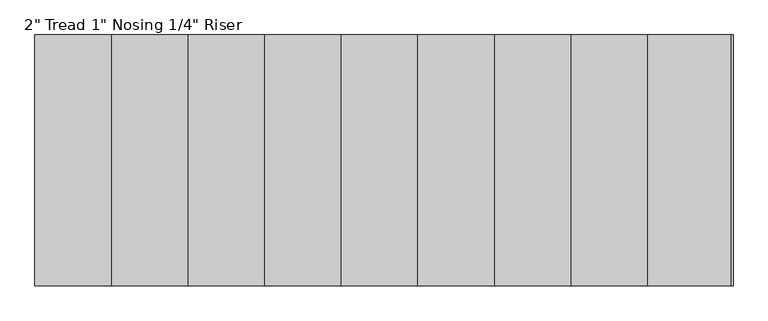
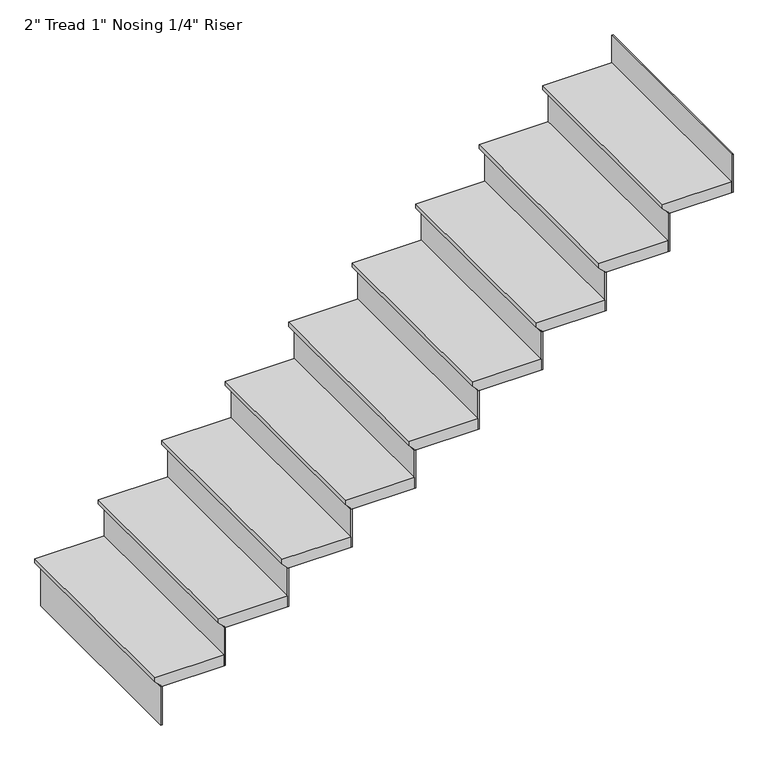
"""IFC4 building model written with IfcOpenShell, lengths in millimetres: stair flight geometry."""

from ifc_helpers import new_model, si_unit, frame, origin, place, context, project, spatial, polyline, outline, extrude, source, transform, mapped, element, save


def stair_flight_9ab9eb73(model_context):
    return source(origin(), model_context, "Body", "SweptSolid", [
        extrude(outline(polyline([(5410.2, 29868.2316163), (5410.2, 29563.4316163), (5391.15, 29563.4316163), (5365.75, 29588.8316163), (5359.4, 29588.8316163), (5359.4, 29868.2316163), (5410.2, 29868.2316163)])), frame((0.0, 7040.8480552, 0.0), z_axis=(0.0, 1.0, 0.0), x_axis=(0.0, 0.0, 1.0)), (0.0, 0.0, 1.0), 914.4),
        extrude(outline(polyline([(29595.1816163, 7040.8480552), (29588.8316163, 7040.8480552), (29588.8316163, 7955.2480552), (29595.1816163, 7955.2480552), (29595.1816163, 7040.8480552)])), frame((0.0, 0.0, 5181.6), z_axis=(0.0, 0.0, 1.0), x_axis=(1.0, 0.0, 0.0)), (0.0, 0.0, 1.0), 177.8),
        extrude(outline(polyline([(29874.5816163, 7040.8480552), (29868.2316163, 7040.8480552), (29868.2316163, 7955.2480552), (29874.5816163, 7955.2480552), (29874.5816163, 7040.8480552)])), frame((0.0, 0.0, 5359.4), z_axis=(0.0, 0.0, 1.0), x_axis=(1.0, 0.0, 0.0)), (0.0, 0.0, 1.0), 177.8),
        extrude(outline(polyline([(5588.0, 30147.6316163), (5588.0, 29842.8316163), (5568.95, 29842.8316163), (5543.55, 29868.2316163), (5537.2, 29868.2316163), (5537.2, 30147.6316163), (5588.0, 30147.6316163)])), frame((0.0, 7040.8480552, 0.0), z_axis=(0.0, 1.0, 0.0), x_axis=(0.0, 0.0, 1.0)), (0.0, 0.0, 1.0), 914.4),
        extrude(outline(polyline([(30153.9816163, 7040.8480552), (30147.6316163, 7040.8480552), (30147.6316163, 7955.2480552), (30153.9816163, 7955.2480552), (30153.9816163, 7040.8480552)])), frame((0.0, 0.0, 5537.2), z_axis=(0.0, 0.0, 1.0), x_axis=(1.0, 0.0, 0.0)), (0.0, 0.0, 1.0), 177.8),
        extrude(outline(polyline([(5765.8, 30427.0316163), (5765.8, 30122.2316163), (5746.75, 30122.2316163), (5721.35, 30147.6316163), (5715.0, 30147.6316163), (5715.0, 30427.0316163), (5765.8, 30427.0316163)])), frame((0.0, 7040.8480552, 0.0), z_axis=(0.0, 1.0, 0.0), x_axis=(0.0, 0.0, 1.0)), (0.0, 0.0, 1.0), 914.4),
        extrude(outline(polyline([(30433.3816163, 7040.8480552), (30427.0316163, 7040.8480552), (30427.0316163, 7955.2480552), (30433.3816163, 7955.2480552), (30433.3816163, 7040.8480552)])), frame((0.0, 0.0, 5715.0), z_axis=(0.0, 0.0, 1.0), x_axis=(1.0, 0.0, 0.0)), (0.0, 0.0, 1.0), 177.8),
        extrude(outline(polyline([(5943.6, 30706.4316163), (5943.6, 30401.6316163), (5924.55, 30401.6316163), (5899.15, 30427.0316163), (5892.8, 30427.0316163), (5892.8, 30706.4316163), (5943.6, 30706.4316163)])), frame((0.0, 7040.8480552, 0.0), z_axis=(0.0, 1.0, 0.0), x_axis=(0.0, 0.0, 1.0)), (0.0, 0.0, 1.0), 914.4),
        extrude(outline(polyline([(30712.7816163, 7040.8480552), (30706.4316163, 7040.8480552), (30706.4316163, 7955.2480552), (30712.7816163, 7955.2480552), (30712.7816163, 7040.8480552)])), frame((0.0, 0.0, 5892.8), z_axis=(0.0, 0.0, 1.0), x_axis=(1.0, 0.0, 0.0)), (0.0, 0.0, 1.0), 177.8),
        extrude(outline(polyline([(6121.4, 30985.8316163), (6121.4, 30681.0316163), (6102.35, 30681.0316163), (6076.95, 30706.4316163), (6070.6, 30706.4316163), (6070.6, 30985.8316163), (6121.4, 30985.8316163)])), frame((0.0, 7040.8480552, 0.0), z_axis=(0.0, 1.0, 0.0), x_axis=(0.0, 0.0, 1.0)), (0.0, 0.0, 1.0), 914.4),
        extrude(outline(polyline([(30992.1816163, 7040.8480552), (30985.8316163, 7040.8480552), (30985.8316163, 7955.2480552), (30992.1816163, 7955.2480552), (30992.1816163, 7040.8480552)])), frame((0.0, 0.0, 6070.6), z_axis=(0.0, 0.0, 1.0), x_axis=(1.0, 0.0, 0.0)), (0.0, 0.0, 1.0), 177.8),
        extrude(outline(polyline([(6299.2, 31265.2316163), (6299.2, 30960.4316163), (6280.15, 30960.4316163), (6254.75, 30985.8316163), (6248.4, 30985.8316163), (6248.4, 31265.2316163), (6299.2, 31265.2316163)])), frame((0.0, 7040.8480552, 0.0), z_axis=(0.0, 1.0, 0.0), x_axis=(0.0, 0.0, 1.0)), (0.0, 0.0, 1.0), 914.4),
        extrude(outline(polyline([(31271.5816163, 7040.8480552), (31265.2316163, 7040.8480552), (31265.2316163, 7955.2480552), (31271.5816163, 7955.2480552), (31271.5816163, 7040.8480552)])), frame((0.0, 0.0, 6248.4), z_axis=(0.0, 0.0, 1.0), x_axis=(1.0, 0.0, 0.0)), (0.0, 0.0, 1.0), 177.8),
        extrude(outline(polyline([(6477.0, 31544.6316163), (6477.0, 31239.8316163), (6457.95, 31239.8316163), (6432.55, 31265.2316163), (6426.2, 31265.2316163), (6426.2, 31544.6316163), (6477.0, 31544.6316163)])), frame((0.0, 7040.8480552, 0.0), z_axis=(0.0, 1.0, 0.0), x_axis=(0.0, 0.0, 1.0)), (0.0, 0.0, 1.0), 914.4),
        extrude(outline(polyline([(31550.9816163, 7040.8480552), (31544.6316163, 7040.8480552), (31544.6316163, 7955.2480552), (31550.9816163, 7955.2480552), (31550.9816163, 7040.8480552)])), frame((0.0, 0.0, 6426.2), z_axis=(0.0, 0.0, 1.0), x_axis=(1.0, 0.0, 0.0)), (0.0, 0.0, 1.0), 177.8),
        extrude(outline(polyline([(6654.8, 31824.0316163), (6654.8, 31519.2316163), (6635.75, 31519.2316163), (6610.35, 31544.6316163), (6604.0, 31544.6316163), (6604.0, 31824.0316163), (6654.8, 31824.0316163)])), frame((0.0, 7040.8480552, 0.0), z_axis=(0.0, 1.0, 0.0), x_axis=(0.0, 0.0, 1.0)), (0.0, 0.0, 1.0), 914.4),
        extrude(outline(polyline([(31830.3816163, 7040.8480552), (31824.0316163, 7040.8480552), (31824.0316163, 7955.2480552), (31830.3816163, 7955.2480552), (31830.3816163, 7040.8480552)])), frame((0.0, 0.0, 6604.0), z_axis=(0.0, 0.0, 1.0), x_axis=(1.0, 0.0, 0.0)), (0.0, 0.0, 1.0), 177.8),
        extrude(outline(polyline([(32109.7816163, 7040.8480552), (32103.4316163, 7040.8480552), (32103.4316163, 7955.2480552), (32109.7816163, 7955.2480552), (32109.7816163, 7040.8480552)])), frame((0.0, 0.0, 6781.8), z_axis=(0.0, 0.0, 1.0), x_axis=(1.0, 0.0, 0.0)), (0.0, 0.0, 1.0), 177.8),
        extrude(outline(polyline([(6832.6, 32103.4316163), (6832.6, 31798.6316163), (6813.55, 31798.6316163), (6788.15, 31824.0316163), (6781.8, 31824.0316163), (6781.8, 32103.4316163), (6832.6, 32103.4316163)])), frame((0.0, 7040.8480552, 0.0), z_axis=(0.0, 1.0, 0.0), x_axis=(0.0, 0.0, 1.0)), (0.0, 0.0, 1.0), 914.4),
    ])


if __name__ == "__main__":
    model = new_model("IFC4")
    model_context = context("Model", 3, world=origin())
    ifc_project = project(units=[si_unit("LENGTHUNIT", "METRE", prefix="MILLI")], contexts=[model_context])
    site = spatial("IfcSite", under=ifc_project)
    building = spatial("IfcBuilding", under=site)
    placement = place(None, origin())
    stair_flight_shape = stair_flight_9ab9eb73(model_context)
    element("IfcStairFlight", 1, ObjectType="2\" Tread 1\" Nosing 1/4\" Riser", at=placement, inside=building, context=model_context, shape_type="MappedRepresentation", body=[
        mapped(stair_flight_shape, transform((0.0, 0.0, 0.0), x_axis=(1.0, 0.0, 0.0), y_axis=(0.0, 1.0, 0.0), z_axis=(0.0, 0.0, 1.0))),
    ])
    save(model, "model.ifc")
